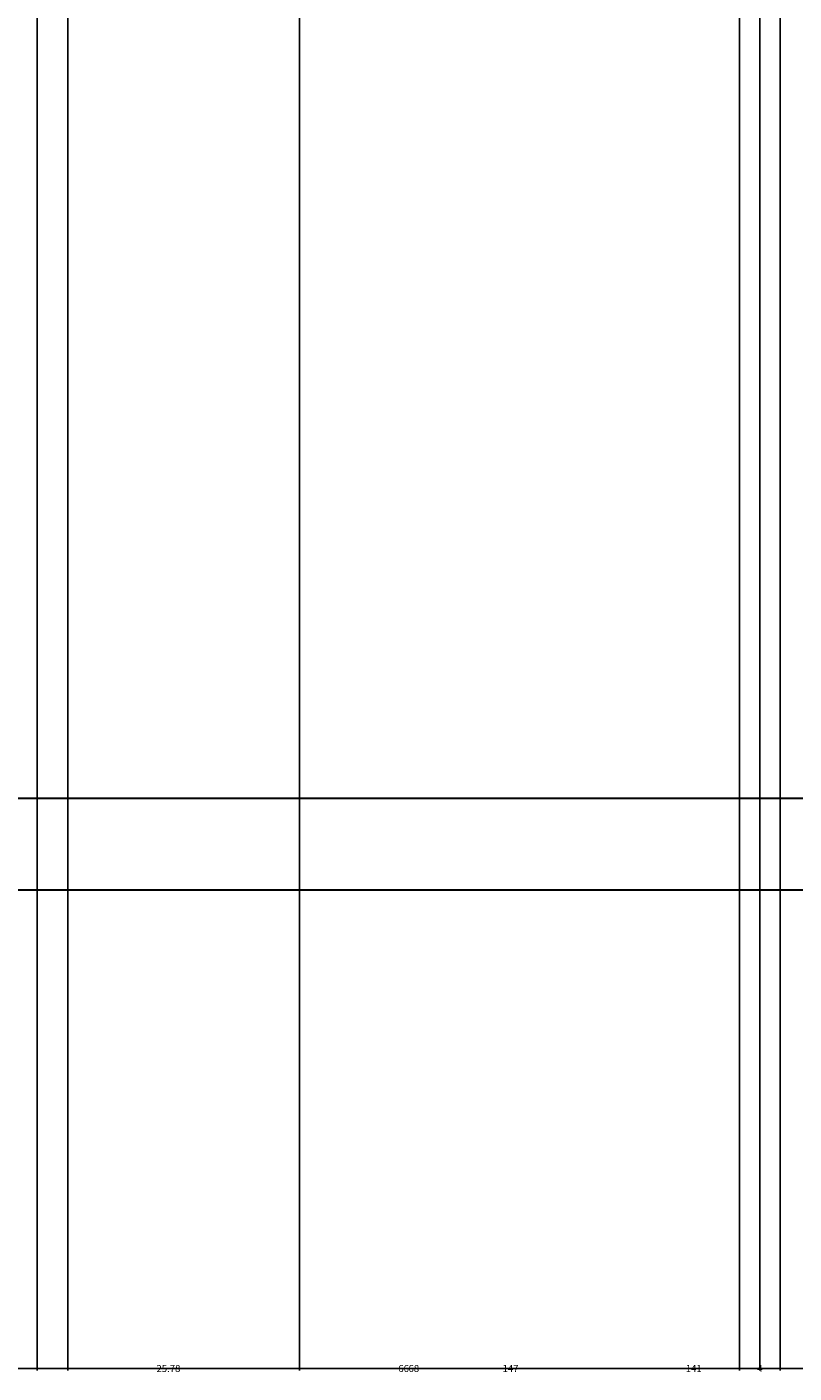
# Model space of a CAD drawing. Units: inches. Extents: x 867 to 1667, y -234 to 788.
# Tile 4 of 42: x 1076 to 1151, y -234 to -102. Entities that reach past the tile are written whole.
import ezdxf

# ---------------------------------------------------------------- set-up
doc = ezdxf.new("R2010")
doc.units = ezdxf.units.IN
doc.header["$MEASUREMENT"] = 0
doc.layers.add('A-ANNO-DIMS', color=2, linetype='Continuous', lineweight=18)
doc.layers.add('A-WALL-SITE', color=8, linetype='Continuous', lineweight=30)
doc.styles.get("Standard").update_dxf_attribs({"font": 'arial.ttf'})
doc.dimstyles.get("Standard").update_dxf_attribs({"dimtxt": 0.6875, "dimasz": 0.18, "dimexe": 0.18, "dimexo": 0.0625, "dimgap": 0.09, "dimtad": 0, "dimdec": 4, "dimzin": 0, "dimdsep": 46, "dimlunit": 4, "dimtxsty": 'Standard', "dimcen": 0.09, "dimadec": 0, "dimazin": 0, "dimtfac": 1, "dimtdec": 4, "dimtofl": 0, "dimtmove": 0, "dimatfit": 3, "dimfxl": 1, "dimtolj": 1, "dimtzin": 0, "dimarcsym": 0})

# ---------------------------------------------------------------- blocks, each defined once
blk = doc.blocks.new('*D27')
at = {"layer": 'A-ANNO-DIMS', "color": 0, "lineweight": -2, "transparency": 16777216}
for p, q in [((1070.89, -55.97), (1070.89, -233.54)), ((1525.26, -186.47), (1525.26, -233.54)), ((1071.07, -233.36), (1296.81, -233.36)), ((1525.08, -233.36), (1299.34, -233.36))]:
    blk.add_line(p, q, dxfattribs=at)
at = {"layer": 'A-ANNO-DIMS', "color": 0, "transparency": 16777216}
for points in [[(1071.07, -233.33), (1071.07, -233.39), (1070.89, -233.36)], [(1525.08, -233.33), (1525.08, -233.39), (1525.26, -233.36)]]:
    blk.add_solid(points, dxfattribs=at)
at = {"layer": 'Defpoints', "color": 0, "transparency": 16777216}
for p in [(1070.89, -55.91), (1525.26, -186.41), (1525.26, -233.36)]:
    blk.add_point(p, dxfattribs=at)
at = {"layer": 'A-ANNO-DIMS', "color": 0, "transparency": 16777216, "insert": (1298.08, -233.36), "char_height": 0.688, "attachment_point": 5}
blk.add_mtext('\\A1;454.4', dxfattribs=at)
blk = doc.blocks.new('*D29')
at = {"layer": 'A-ANNO-DIMS', "color": 0, "lineweight": -2, "transparency": 16777216}
for p, q in [((1076.89, 623.55), (1076.89, -233.54)), ((1102.67, 623.55), (1102.67, -233.54)), ((1077.07, -233.36), (1088.52, -233.36)), ((1102.49, -233.36), (1091.03, -233.36))]:
    blk.add_line(p, q, dxfattribs=at)
at = {"layer": 'A-ANNO-DIMS', "color": 0, "transparency": 16777216}
for points in [[(1077.07, -233.33), (1077.07, -233.39), (1076.89, -233.36)], [(1102.49, -233.33), (1102.49, -233.39), (1102.67, -233.36)]]:
    blk.add_solid(points, dxfattribs=at)
at = {"layer": 'Defpoints', "color": 0, "transparency": 16777216}
for p in [(1076.89, 623.62), (1102.67, 623.62), (1102.67, -233.36)]:
    blk.add_point(p, dxfattribs=at)
at = {"layer": 'A-ANNO-DIMS', "color": 0, "transparency": 16777216, "insert": (1089.78, -233.36), "char_height": 0.688, "attachment_point": 5}
blk.add_mtext('\\A1;25.78', dxfattribs=at)
blk = doc.blocks.new('*D37')
at = {"layer": 'A-ANNO-DIMS', "color": 0, "lineweight": -2, "transparency": 16777216}
for p, q in [((1049.89, 257.55), (1049.89, -233.54)), ((1196.89, 257.55), (1196.89, -233.54)), ((1050.07, -233.36), (1122.57, -233.36)), ((1196.71, -233.36), (1124.2, -233.36))]:
    blk.add_line(p, q, dxfattribs=at)
at = {"layer": 'A-ANNO-DIMS', "color": 0, "transparency": 16777216}
for points in [[(1050.07, -233.33), (1050.07, -233.39), (1049.89, -233.36)], [(1196.71, -233.33), (1196.71, -233.39), (1196.89, -233.36)]]:
    blk.add_solid(points, dxfattribs=at)
at = {"layer": 'Defpoints', "color": 0, "transparency": 16777216}
for p in [(1049.89, 257.62), (1196.89, 257.62), (1196.89, -233.36)]:
    blk.add_point(p, dxfattribs=at)
at = {"layer": 'A-ANNO-DIMS', "color": 0, "transparency": 16777216, "insert": (1123.39, -233.36), "char_height": 0.688, "attachment_point": 5}
blk.add_mtext('\\A1;147', dxfattribs=at)
blk = doc.blocks.new('*D42')
at = {"layer": 'A-ANNO-DIMS', "color": 0, "lineweight": -2, "transparency": 16777216}
for p, q in [((1079.89, 136.05), (1079.89, -233.54)), ((1145.89, 136.05), (1145.89, -233.54)), ((1080.07, -233.36), (1112.3, -233.36)), ((1145.71, -233.36), (1113.47, -233.36))]:
    blk.add_line(p, q, dxfattribs=at)
at = {"layer": 'A-ANNO-DIMS', "color": 0, "transparency": 16777216}
for points in [[(1080.07, -233.33), (1080.07, -233.39), (1079.89, -233.36)], [(1145.71, -233.33), (1145.71, -233.39), (1145.89, -233.36)]]:
    blk.add_solid(points, dxfattribs=at)
at = {"layer": 'Defpoints', "color": 0, "transparency": 16777216}
for p in [(1079.89, 136.12), (1145.89, 136.12), (1145.89, -233.36)]:
    blk.add_point(p, dxfattribs=at)
at = {"layer": 'A-ANNO-DIMS', "color": 0, "transparency": 16777216, "insert": (1112.89, -233.36), "char_height": 0.688, "attachment_point": 5}
blk.add_mtext('\\A1;66', dxfattribs=at)
blk = doc.blocks.new('*D43')
at = {"layer": 'A-ANNO-DIMS', "color": 0, "lineweight": -2, "transparency": 16777216}
for p, q in [((1145.89, 136.05), (1145.89, -233.54)), ((1149.89, 136.05), (1149.89, -233.54)), ((1146.07, -233.36), (1147.56, -233.36)), ((1149.71, -233.36), (1148.21, -233.36))]:
    blk.add_line(p, q, dxfattribs=at)
at = {"layer": 'A-ANNO-DIMS', "color": 0, "transparency": 16777216}
for points in [[(1146.07, -233.33), (1146.07, -233.39), (1145.89, -233.36)], [(1149.71, -233.33), (1149.71, -233.39), (1149.89, -233.36)]]:
    blk.add_solid(points, dxfattribs=at)
at = {"layer": 'Defpoints', "color": 0, "transparency": 16777216}
for p in [(1145.89, 136.12), (1149.89, 136.12), (1149.89, -233.36)]:
    blk.add_point(p, dxfattribs=at)
at = {"layer": 'A-ANNO-DIMS', "color": 0, "transparency": 16777216, "insert": (1147.89, -233.36), "char_height": 0.688, "attachment_point": 5}
blk.add_mtext('\\A1;4', dxfattribs=at)
blk = doc.blocks.new('*D45')
at = {"layer": 'A-ANNO-DIMS', "color": 0, "lineweight": -2, "transparency": 16777216}
for p, q in [((1079.89, -7.95), (1079.89, -233.54)), ((1247.89, -7.95), (1247.89, -233.54)), ((1080.07, -233.36), (1163.07, -233.36)), ((1247.71, -233.36), (1164.7, -233.36))]:
    blk.add_line(p, q, dxfattribs=at)
at = {"layer": 'A-ANNO-DIMS', "color": 0, "transparency": 16777216}
for points in [[(1080.07, -233.33), (1080.07, -233.39), (1079.89, -233.36)], [(1247.71, -233.33), (1247.71, -233.39), (1247.89, -233.36)]]:
    blk.add_solid(points, dxfattribs=at)
at = {"layer": 'Defpoints', "color": 0, "transparency": 16777216}
for p in [(1079.89, -7.88), (1247.89, -7.88), (1247.89, -233.36)]:
    blk.add_point(p, dxfattribs=at)
at = {"layer": 'A-ANNO-DIMS', "color": 0, "transparency": 16777216, "insert": (1163.89, -233.36), "char_height": 0.688, "attachment_point": 5}
blk.add_mtext('\\A1;168', dxfattribs=at)
blk = doc.blocks.new('*D49')
at = {"layer": 'A-ANNO-DIMS', "color": 0, "lineweight": -2, "transparency": 16777216}
for p, q in [((1070.89, -55.97), (1070.89, -233.54)), ((1211.89, -55.97), (1211.89, -233.54)), ((1071.07, -233.36), (1140.64, -233.36)), ((1211.71, -233.36), (1142.14, -233.36))]:
    blk.add_line(p, q, dxfattribs=at)
at = {"layer": 'A-ANNO-DIMS', "color": 0, "transparency": 16777216}
for points in [[(1071.07, -233.33), (1071.07, -233.39), (1070.89, -233.36)], [(1211.71, -233.33), (1211.71, -233.39), (1211.89, -233.36)]]:
    blk.add_solid(points, dxfattribs=at)
at = {"layer": 'Defpoints', "color": 0, "transparency": 16777216}
for p in [(1070.89, -55.91), (1211.89, -55.91), (1211.89, -233.36)]:
    blk.add_point(p, dxfattribs=at)
at = {"layer": 'A-ANNO-DIMS', "color": 0, "transparency": 16777216, "insert": (1141.39, -233.36), "char_height": 0.688, "attachment_point": 5}
blk.add_mtext('\\A1;141', dxfattribs=at)
blk = doc.blocks.new('*D57')
at = {"layer": 'A-ANNO-DIMS', "color": 0, "lineweight": -2, "transparency": 16777216}
for p, q in [((1079.89, -7.95), (1079.89, -233.54)), ((1147.89, -7.95), (1147.89, -233.54)), ((1080.07, -233.36), (1113.3, -233.36)), ((1147.71, -233.36), (1114.47, -233.36))]:
    blk.add_line(p, q, dxfattribs=at)
at = {"layer": 'A-ANNO-DIMS', "color": 0, "transparency": 16777216}
for points in [[(1080.07, -233.33), (1080.07, -233.39), (1079.89, -233.36)], [(1147.71, -233.33), (1147.71, -233.39), (1147.89, -233.36)]]:
    blk.add_solid(points, dxfattribs=at)
at = {"layer": 'Defpoints', "color": 0, "transparency": 16777216}
for p in [(1079.89, -7.88), (1147.89, -7.88), (1147.89, -233.36)]:
    blk.add_point(p, dxfattribs=at)
at = {"layer": 'A-ANNO-DIMS', "color": 0, "transparency": 16777216, "insert": (1113.89, -233.36), "char_height": 0.688, "attachment_point": 5}
blk.add_mtext('\\A1;68', dxfattribs=at)

msp = doc.modelspace()

# ---------------------------------------------------------------- linework, layer by layer
at = {"layer": 'A-WALL-SITE'}
for p, q in [((1526.8389, -177.4081), (1006.3882, -177.4081)), ((1619.8866, -186.4081), (914.8866, -186.4081))]:
    msp.add_line(p, q, dxfattribs=at)

# ---------------------------------------------------------------- dimensions: what is measured, and where the dimension line sits
at = {"layer": 'A-ANNO-DIMS'}
for base, p1, p2, override, picture, middle in [((1102.6661, -233.3581), (1076.8866, 623.617), (1102.6661, 623.617), {"dimdec": 2, "dimlfac": 1, "dimrnd": 0, "dimzin": 0, "dimdsep": 46, "dimlunit": 2}, '*D29', (1089.7763, -233.3581)), ((1196.8866, -233.3581), (1049.8866, 257.617), (1196.8866, 257.617), {"dimdec": 0, "dimlfac": 1, "dimrnd": 0, "dimzin": 0, "dimdsep": 46, "dimlunit": 2}, '*D37', (1123.3866, -233.3581)), ((1145.8866, -233.3581), (1079.8866, 136.117), (1145.8866, 136.117), {"dimdec": 0, "dimlfac": 1, "dimrnd": 0, "dimzin": 0, "dimdsep": 46, "dimlunit": 2}, '*D42', (1112.8866, -233.3581)), ((1149.8866, -233.3581), (1145.8866, 136.117), (1149.8866, 136.117), {"dimdec": 0, "dimlfac": 1, "dimrnd": 0, "dimzin": 0, "dimdsep": 46, "dimlunit": 2}, '*D43', (1147.8866, -233.3581)), ((1247.8866, -233.3581), (1079.8866, -7.883), (1247.8866, -7.883), {"dimdec": 0, "dimlfac": 1, "dimrnd": 0, "dimzin": 0, "dimdsep": 46, "dimlunit": 2}, '*D45', (1163.8866, -233.3581)), ((1147.8918, -233.3581), (1079.8866, -7.883), (1147.8918, -7.883), {"dimdec": 0, "dimlfac": 1, "dimrnd": 0, "dimzin": 0, "dimdsep": 46, "dimlunit": 2}, '*D57', (1113.8892, -233.3581)), ((1525.2648, -233.3581), (1070.8866, -55.9081), (1525.2648, -186.4081), {"dimdec": 1, "dimlfac": 1, "dimrnd": 0, "dimzin": 0, "dimdsep": 46, "dimlunit": 2}, '*D27', (1298.0757, -233.3581)), ((1211.8866, -233.3581), (1070.8866, -55.9081), (1211.8866, -55.9081), {"dimdec": 0, "dimlfac": 1, "dimrnd": 0, "dimzin": 0, "dimdsep": 46, "dimlunit": 2}, '*D49', (1141.3866, -233.3581))]:
    dim = msp.add_linear_dim(base=base, p1=p1, p2=p2, dimstyle='Standard', override=override, dxfattribs=at)
    dim.commit()
    dim.dimension.update_dxf_attribs({"geometry": picture, "text_midpoint": middle})

doc.saveas('drawing.dxf')
